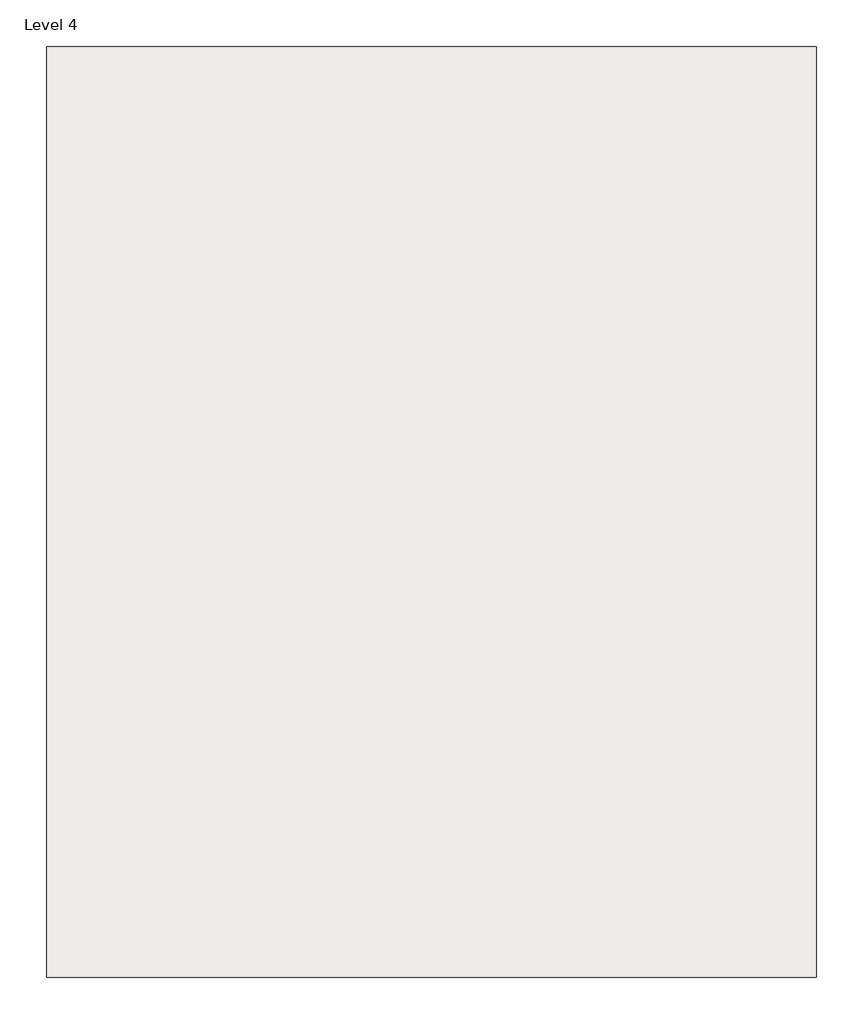
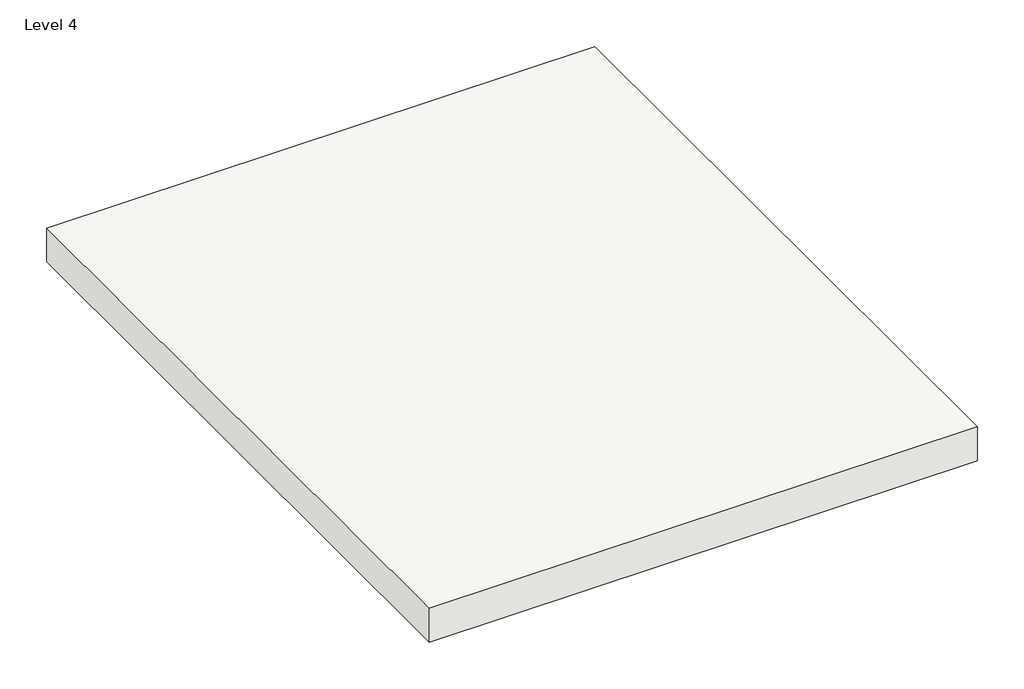
# One storey: 1 roof.
"""IFC4 building model written with IfcOpenShell, lengths in millimetres."""

from ifc_helpers import new_model, si_unit, frame, origin, place, context, project, spatial, polyline, outline, extrude, element, save

model = new_model("IFC4")

# Units and contexts
model_context = context("Model", 3, world=origin())
ifc_project = project(units=[si_unit("LENGTHUNIT", "METRE", prefix="MILLI")], contexts=[model_context])

# Site, building, storey
site = spatial("IfcSite", under=ifc_project)
building = spatial("IfcBuilding", under=site)
storey = spatial("IfcBuildingStorey", under=building, Name="Level 4", Elevation=10972.8)

# Roof
placement = place(None, origin())
element("IfcRoof", 1, ObjectType="Generic - 12\"", at=placement, inside=storey, context=model_context, shape_type="SweptSolid", body=[
    extrude(outline(polyline([(-12021.6009794, 2760.6416393), (-7341.2932708, 2760.6416393), (-7341.2932708, -2901.4387205), (-12021.6009794, -2901.4387205), (-12021.6009794, 2760.6416393)])), frame((0.0, 0.0, 10972.8), z_axis=(0.0, 0.0, 1.0), x_axis=(1.0, 0.0, 0.0)), (0.0, 0.0, 1.0), 304.8),
])

save(model, "model.ifc")

# Revit data of these elements
# Type "Generic - 12\""
#   Assembly Code = "B1020"
#   Layers, outside or top first: 1' - 0" no material (function 1)
# Element 1 (IfcRoof, "Generic - 12\"")
#   built-in parameter 1001705 = 37 (stored number, unit not read)
#   built-in parameter 1001710 = 33615
#   Phase Created = New Construction
#   Materials on its faces: "Default Roof"
# Materials
#   "Default Roof": colour RGB 88 101 114, transparency 0
